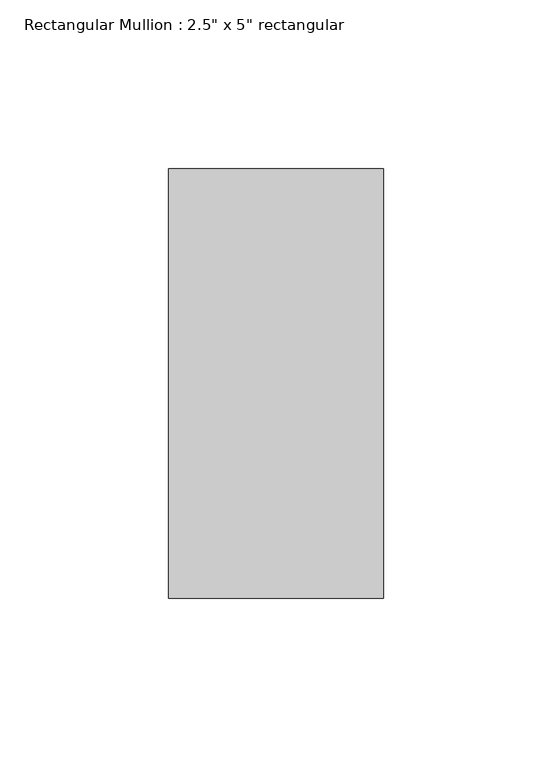
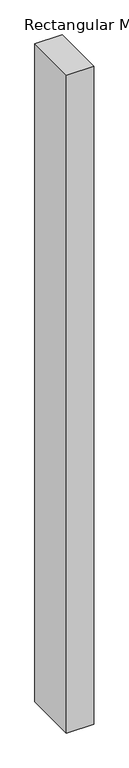
"""IFC4 building model written with IfcOpenShell, lengths in millimetres: member geometry."""

from ifc_helpers import new_model, si_unit, frame, origin, place, context, project, spatial, polyline, outline, extrude, source, transform, mapped, element, save


def member_cf38170e(model_context):
    return source(origin(), model_context, "Body", "SweptSolid", [
        extrude(outline(polyline([(0.0, 63.5), (0.0, -63.5), (-63.5, -63.5), (-63.5, 63.5), (0.0, 63.5)])), frame((0.0, 0.0, -1619.7840707), z_axis=(0.0, 0.0, 1.0), x_axis=(1.0, 0.0, 0.0)), (0.0, 0.0, 1.0), 1619.7840707),
    ])


if __name__ == "__main__":
    model = new_model("IFC4")
    model_context = context("Model", 3, world=origin())
    ifc_project = project(units=[si_unit("LENGTHUNIT", "METRE", prefix="MILLI")], contexts=[model_context])
    site = spatial("IfcSite", under=ifc_project)
    building = spatial("IfcBuilding", under=site)
    placement = place(None, origin())
    member_shape = member_cf38170e(model_context)
    element("IfcMember", 1, ObjectType="Rectangular Mullion : 2.5\" x 5\" rectangular", at=placement, inside=building, context=model_context, shape_type="MappedRepresentation", body=[
        mapped(member_shape, transform((0.0, 0.0, 0.0), x_axis=(1.0, 0.0, 0.0), y_axis=(0.0, 1.0, 0.0), z_axis=(0.0, 0.0, 1.0))),
    ])
    save(model, "model.ifc")

# Revit data of these elements
# Type "Rectangular Mullion : 2.5\" x 5\" rectangular"
#   built-in parameter 1007304 = 0.416667 (stored number, unit not read)
#   built-in parameter 1007301 = 0.104167 (stored number, unit not read)
#   built-in parameter 1007300 = 0.104167 (stored number, unit not read)
# Element 1 (IfcMember, "Rectangular Mullion : 2.5\" x 5\" rectangular")
#   Materials on its faces: "Aluminum"
# Materials
#   "Aluminum": class "Metal", colour RGB 247 247 247, transparency 0, Description = "Aluminum 6061", Cost = 0
